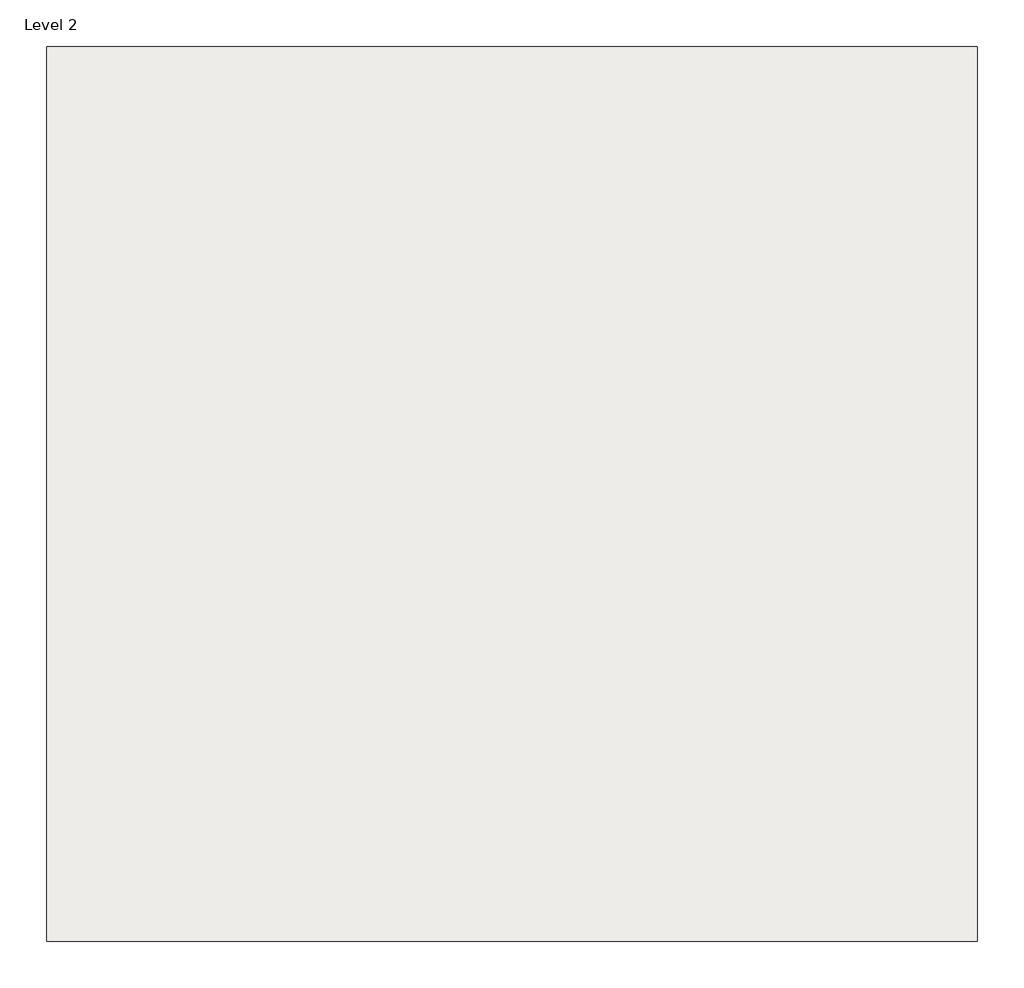
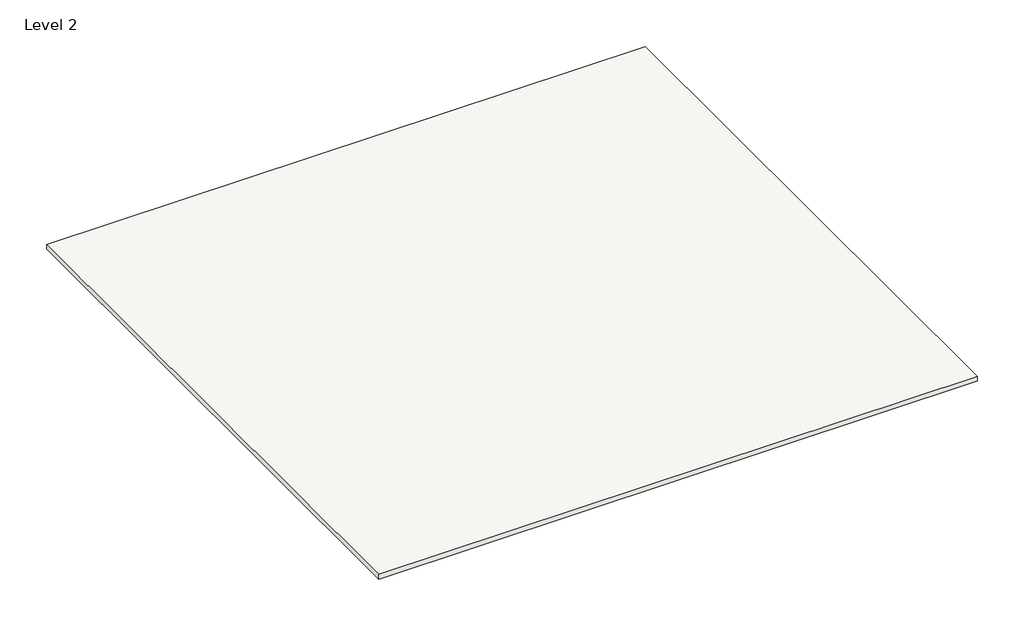
# One storey: 1 slab.
"""IFC4 building model written with IfcOpenShell, lengths in millimetres."""

from ifc_helpers import new_model, si_unit, frame, origin, place, context, project, spatial, polyline, outline, extrude, element, save

model = new_model("IFC4")

# Units and contexts
model_context = context("Model", 3, world=origin())
ifc_project = project(units=[si_unit("LENGTHUNIT", "METRE", prefix="MILLI")], contexts=[model_context])

# Site, building, storey
site = spatial("IfcSite", under=ifc_project)
building = spatial("IfcBuilding", under=site)
storey = spatial("IfcBuildingStorey", under=building, Name="Level 2", Elevation=3657.6)

# Slab
placement = place(None, origin())
element("IfcSlab", 1, ObjectType="6\" floor", at=placement, inside=storey, context=model_context, shape_type="SweptSolid", body=[
    extrude(outline(polyline([(8746.1579341, 8977.7121658), (8746.1579341, -8827.6878342), (-9770.4420659, -8827.6878342), (-9770.4420659, 8977.7121658), (8746.1579341, 8977.7121658)])), frame((0.0, 0.0, 3657.6), z_axis=(0.0, 0.0, 1.0), x_axis=(1.0, 0.0, 0.0)), (0.0, 0.0, 1.0), 152.4),
])

save(model, "model.ifc")

# Revit data of these elements
# Type "6\" floor"
#   Assembly Code = "B1010"
#   Function = 0
#   Layers, outside or top first: 0' - 6" no material (function 1)
# Element 1 (IfcSlab, "6\" floor")
#   Height Offset From Level = 0' - 6"
#   Phase Created = New Construction
#   Materials on its faces: "Default Floor"
# Materials
#   "Default Floor": colour RGB 128 128 128, transparency 0, Cost = 0
